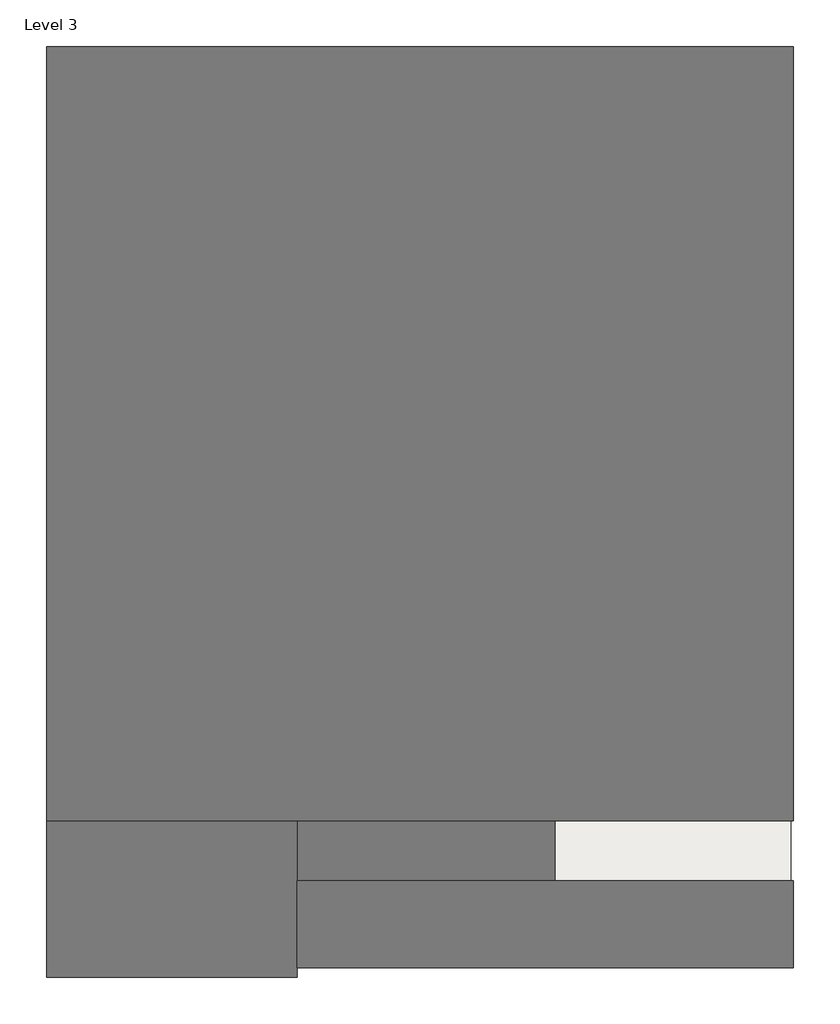
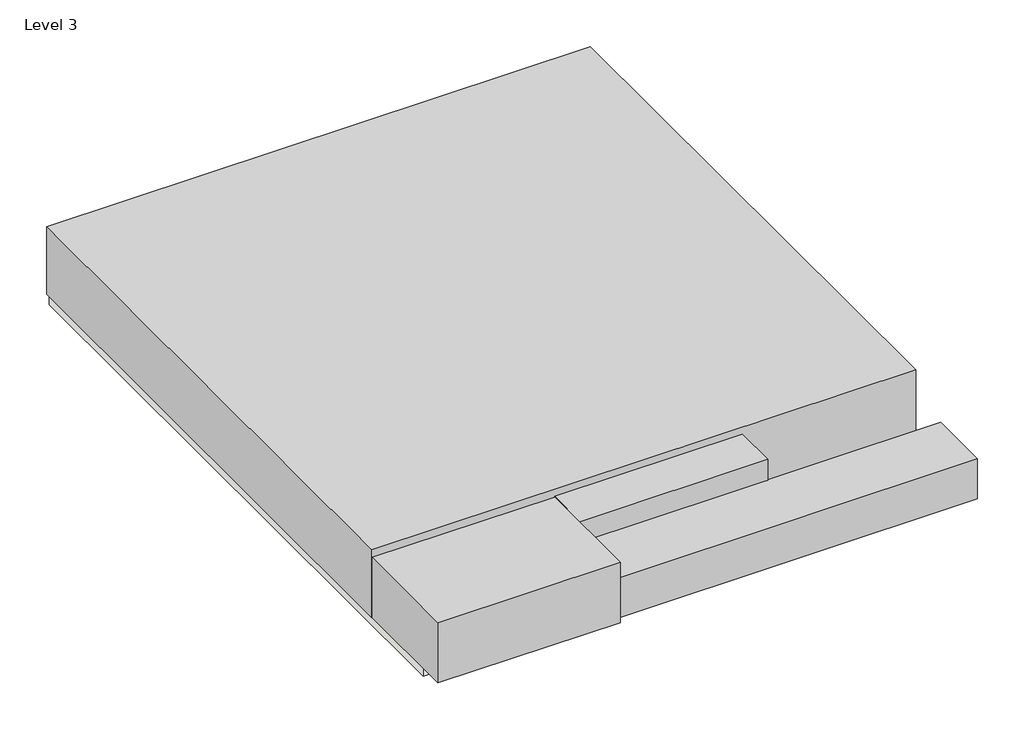
# One storey: 4 proxies, 1 roof.
"""IFC4 building model written with IfcOpenShell, lengths in millimetres."""

from ifc_helpers import new_model, si_unit, frame, origin, place, context, project, spatial, polyline, outline, extrude, transform, mapped, element, save
from components import generic_models_1_generic_models_1_82b812d9, generic_models_2_generic_models_2_5ecfa4da, generic_models_3_generic_models_3_d114d96d, generic_models_5_generic_models_5_907641ea

model = new_model("IFC4")

# Units and contexts
model_context = context("Model", 3, world=origin())
ifc_project = project(units=[si_unit("LENGTHUNIT", "METRE", prefix="MILLI")], contexts=[model_context])

# Site, building, storey
site = spatial("IfcSite", under=ifc_project)
building = spatial("IfcBuilding", under=site)
storey = spatial("IfcBuildingStorey", under=building, Name="Level 3", Elevation=6096.0)

# Proxies
placement = place(None, origin())
generic_models_1_generic_models_1_shape = generic_models_1_generic_models_1_82b812d9(model_context)
element("IfcBuildingElementProxy", 1, Name="Generic Models 1 : Generic Models 1", ObjectType="Generic Models 1 : Generic Models 1", at=placement, inside=storey, context=model_context, shape_type="MappedRepresentation", body=[
    mapped(generic_models_1_generic_models_1_shape, transform((0.0, 0.0, 0.0), x_axis=(1.0, 0.0, 0.0), y_axis=(0.0, 1.0, 0.0), z_axis=(0.0, 0.0, 1.0))),
])
generic_models_2_generic_models_2_shape = generic_models_2_generic_models_2_5ecfa4da(model_context)
element("IfcBuildingElementProxy", 2, Name="Generic Models 2 : Generic Models 2", ObjectType="Generic Models 2 : Generic Models 2", at=placement, inside=storey, context=model_context, shape_type="MappedRepresentation", body=[
    mapped(generic_models_2_generic_models_2_shape, transform((0.0, 0.0, 0.0), x_axis=(1.0, 0.0, 0.0), y_axis=(0.0, 1.0, 0.0), z_axis=(0.0, 0.0, 1.0))),
])
generic_models_3_generic_models_3_shape = generic_models_3_generic_models_3_d114d96d(model_context)
element("IfcBuildingElementProxy", 3, Name="Generic Models 3 : Generic Models 3", ObjectType="Generic Models 3 : Generic Models 3", at=placement, inside=storey, context=model_context, shape_type="MappedRepresentation", body=[
    mapped(generic_models_3_generic_models_3_shape, transform((0.0, 0.0, 0.0), x_axis=(1.0, 0.0, 0.0), y_axis=(0.0, 1.0, 0.0), z_axis=(0.0, 0.0, 1.0))),
])
generic_models_5_generic_models_5_shape = generic_models_5_generic_models_5_907641ea(model_context)
element("IfcBuildingElementProxy", 4, Name="Generic Models 5 : Generic Models 5", ObjectType="Generic Models 5 : Generic Models 5", at=placement, inside=storey, context=model_context, shape_type="MappedRepresentation", body=[
    mapped(generic_models_5_generic_models_5_shape, transform((0.0, 0.0, 0.0), x_axis=(1.0, 0.0, 0.0), y_axis=(0.0, 1.0, 0.0), z_axis=(0.0, 0.0, 1.0))),
])

# Roof
element("IfcRoof", 5, ObjectType="Generic - 12\"", at=placement, inside=storey, context=model_context, shape_type="SweptSolid", body=[
    extrude(outline(polyline([(-10412.4069895, 9947.6019701), (4929.1930105, 9947.6019701), (4929.1930105, -8441.9980299), (-10412.4069895, -8441.9980299), (-10412.4069895, 9947.6019701)])), frame((0.0, 0.0, 6096.0), z_axis=(0.0, 0.0, 1.0), x_axis=(1.0, 0.0, 0.0)), (0.0, 0.0, 1.0), 304.8),
])

save(model, "model.ifc")

# Revit data of these elements
# Type "Generic - 12\""
#   Assembly Code = "B1020"
#   Layers, outside or top first: 1' - 0" no material (function 1)
# Element 1 (IfcBuildingElementProxy, "Generic Models 1 : Generic Models 1")
#   Phase Created = New Construction
# Element 2 (IfcBuildingElementProxy, "Generic Models 2 : Generic Models 2")
#   Phase Created = New Construction
# Element 3 (IfcBuildingElementProxy, "Generic Models 3 : Generic Models 3")
#   Phase Created = New Construction
# Element 4 (IfcBuildingElementProxy, "Generic Models 5 : Generic Models 5")
#   Phase Created = New Construction
# Element 5 (IfcRoof, "Generic - 12\"")
#   built-in parameter 1001705 = 21 (stored number, unit not read)
#   built-in parameter 1001710 = 33615
#   Phase Created = New Construction
#   Materials on its faces: "Default Roof"
# Materials
#   "Default Roof": colour RGB 88 101 114, transparency 0
